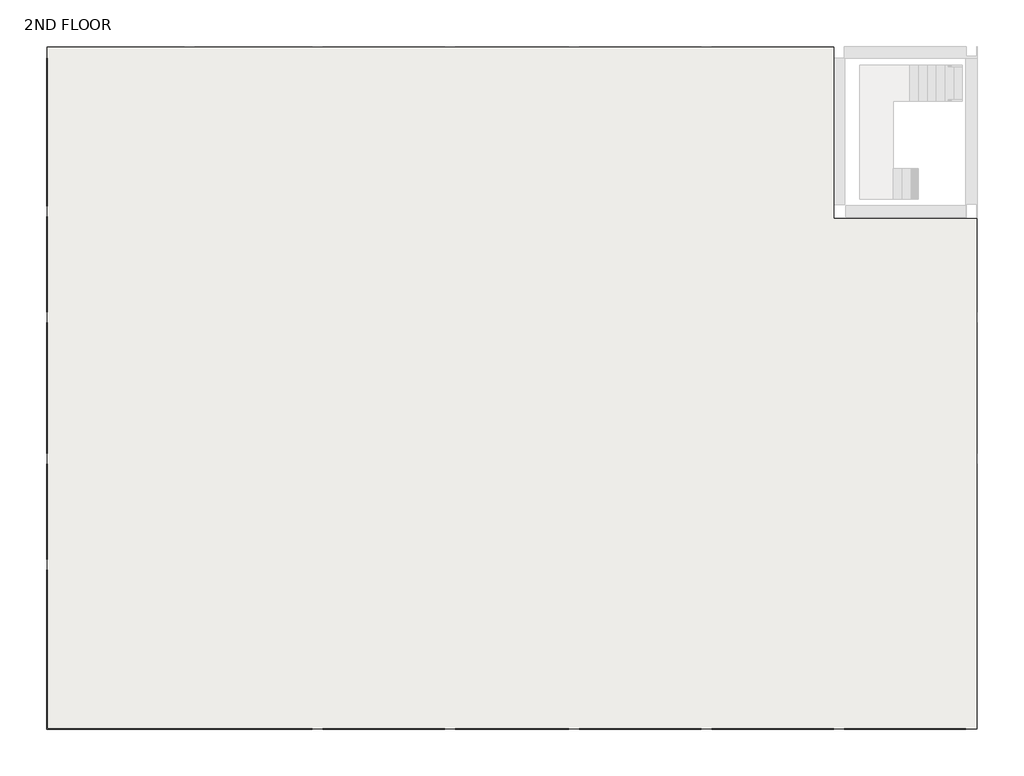
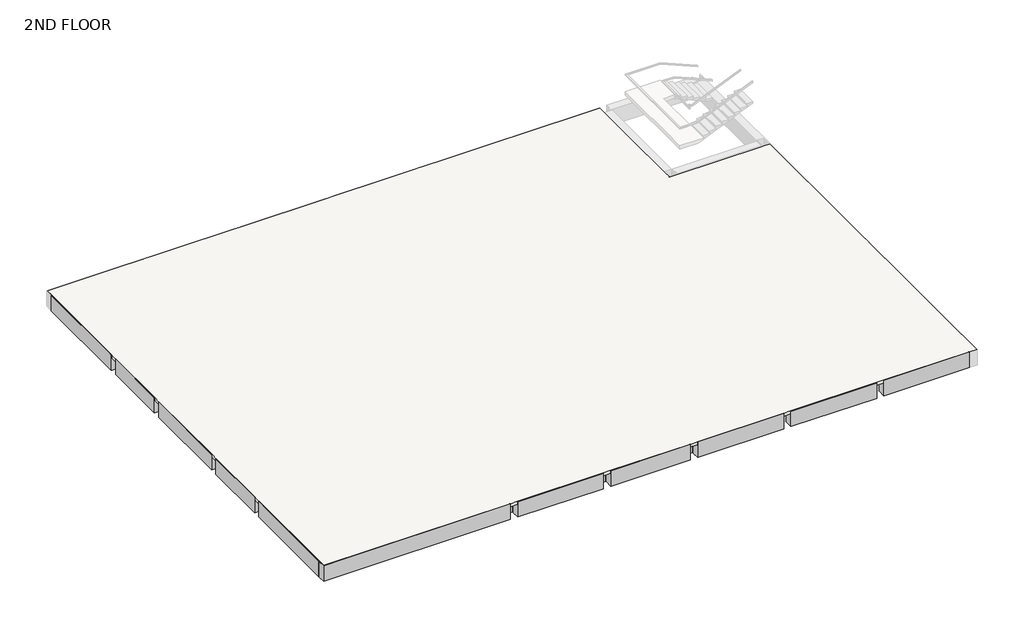
# One storey, part 1 of 2: 9 beams, 1 slab.
"""IFC4 building model written with IfcOpenShell, lengths in millimetres."""

from ifc_helpers import new_model, si_unit, frame, origin, place, context, project, spatial, polyline, outline, extrude, faceted_brep, element, save

model = new_model("IFC4")

# Units and contexts
model_context = context("Model", 3, world=origin())
ifc_project = project(units=[si_unit("LENGTHUNIT", "METRE", prefix="MILLI")], contexts=[model_context])

# Site, building, storey
site = spatial("IfcSite", under=ifc_project)
building = spatial("IfcBuilding", under=site)
storey = spatial("IfcBuildingStorey", under=building, Name="2ND FLOOR", Elevation=7620.0)

# Beams
placement = place(None, origin())
element("IfcBeam", 1, ObjectType="M_Concrete-Rectangular Beam : 400 x 800mm", at=placement, inside=storey, context=model_context, shape_type="Brep", body=[
    faceted_brep([(-25701.5491019, -6047.8309165, 7620.0), (-25701.5491019, -6447.8309165, 7620.0), (-16535.3491019, -6447.8309165, 7620.0), (-16535.3491019, -6425.6309165, 7620.0), (-25679.3491019, -6425.6309165, 7620.0), (-25679.3491019, -6047.8309165, 7620.0), (-25701.5491019, -6047.8309165, 6820.0), (-25679.3491019, -6047.8309165, 7467.6), (-25301.5491019, -6047.8309165, 7467.6), (-20977.1491019, -6047.8309165, 7467.6), (-20577.1491019, -6047.8309165, 7467.6), (-16557.5491019, -6047.8309165, 7467.6), (-16535.3491019, -6047.8309165, 7467.6), (-16535.3491019, -6047.8309165, 6820.0), (-16557.5491019, -6047.8309165, 6820.0), (-20577.1491019, -6047.8309165, 6820.0), (-20977.1491019, -6047.8309165, 6820.0), (-25301.5491019, -6047.8309165, 6820.0), (-25701.5491019, -6447.8309165, 6820.0), (-16535.3491019, -6447.8309165, 6820.0), (-25323.7491019, -6425.6309165, 6820.0), (-25323.7491019, -6070.0309165, 6820.0), (-25679.3491019, -6070.0309165, 6820.0), (-25679.3491019, -6425.6309165, 6820.0), (-20599.3491019, -6425.6309165, 6820.0), (-20599.3491019, -6070.0309165, 6820.0), (-20954.9491019, -6070.0309165, 6820.0), (-20954.9491019, -6425.6309165, 6820.0), (-25323.7491019, -6425.6309165, 7467.6), (-25323.7491019, -6070.0309165, 7467.6), (-16535.3491019, -6425.6309165, 7467.6), (-20599.3491019, -6425.6309165, 7467.6), (-20954.9491019, -6425.6309165, 7467.6), (-25679.3491019, -6425.6309165, 7467.6), (-25679.3491019, -6070.0309165, 7467.6), (-20599.3491019, -6070.0309165, 7467.6), (-20954.9491019, -6070.0309165, 7467.6)], [[[0, 1, 2, 3, 4, 5]], [[6, 0, 5, 7, 8, 9, 10, 11, 12, 13, 14, 15, 16, 17]], [[18, 6, 17, 16, 15, 14, 13, 19], [20, 21, 22, 23], [24, 25, 26, 27]], [[1, 18, 19, 2]], [[1, 0, 6, 18]], [[21, 20, 28, 29]], [[30, 31, 24, 27, 32, 28, 20, 23, 33, 4, 3]], [[4, 33, 23, 22, 34, 7, 5]], [[22, 21, 29, 34]], [[25, 24, 31, 35]], [[27, 26, 36, 32]], [[26, 25, 35, 36]], [[19, 13, 12, 30, 3, 2]], [[28, 32, 36, 35, 31, 30, 12, 11, 10, 9, 8, 7, 34, 29]]]),
    faceted_brep([(5997.6508981, -6447.8309165, 6820.0), (5997.6508981, -6047.8309165, 6820.0), (5997.6508981, -6047.8309165, 7467.6), (5997.6508981, -6425.6309165, 7467.6), (5997.6508981, -6425.6309165, 7620.0), (5997.6508981, -6447.8309165, 7620.0), (1803.4508981, -6047.8309165, 6820.0), (1803.4508981, -6447.8309165, 6820.0), (1803.4508981, -6447.8309165, 7620.0), (1803.4508981, -6425.6309165, 7620.0), (1803.4508981, -6425.6309165, 7467.6), (1803.4508981, -6047.8309165, 7467.6), (1825.6508981, -6047.8309165, 6820.0), (1825.6508981, -6047.8309165, 7467.6)], [[[0, 1, 2, 3, 4, 5]], [[6, 7, 8, 9, 10, 11]], [[8, 5, 4, 9]], [[1, 12, 6, 11, 13, 2]], [[1, 0, 7, 6, 12]], [[0, 5, 8, 7]], [[10, 3, 2, 13, 11]], [[3, 10, 9, 4]]]),
    faceted_brep([(-16179.7491019, -6047.8309165, 6820.0), (-16179.7491019, -6447.8309165, 6820.0), (-16179.7491019, -6447.8309165, 7620.0), (-16179.7491019, -6425.6309165, 7620.0), (-16179.7491019, -6425.6309165, 7467.6), (-16179.7491019, -6047.8309165, 7467.6), (-11963.3491019, -6447.8309165, 7620.0), (-11963.3491019, -6425.6309165, 7620.0), (-11963.3491019, -6047.8309165, 6820.0), (-11985.5491019, -6047.8309165, 6820.0), (-16157.5491019, -6047.8309165, 6820.0), (-16157.5491019, -6047.8309165, 7467.6), (-11985.5491019, -6047.8309165, 7467.6), (-11963.3491019, -6047.8309165, 7467.6), (-11963.3491019, -6447.8309165, 6820.0), (-11963.3491019, -6425.6309165, 7467.6)], [[[0, 1, 2, 3, 4, 5]], [[2, 6, 7, 3]], [[8, 9, 10, 0, 5, 11, 12, 13]], [[1, 0, 10, 9, 8, 14]], [[2, 1, 14, 6]], [[14, 8, 13, 15, 7, 6]], [[15, 4, 3, 7]], [[4, 15, 13, 12, 11, 5]]]),
    faceted_brep([(-11607.7491019, -6047.8309165, 6820.0), (-11607.7491019, -6447.8309165, 6820.0), (-11607.7491019, -6447.8309165, 7620.0), (-11607.7491019, -6425.6309165, 7620.0), (-11607.7491019, -6425.6309165, 7467.6), (-11607.7491019, -6047.8309165, 7467.6), (-7696.1491019, -6447.8309165, 7620.0), (-7696.1491019, -6425.6309165, 7620.0), (-7696.1491019, -6047.8309165, 6820.0), (-7718.3491019, -6047.8309165, 6820.0), (-11585.5491019, -6047.8309165, 6820.0), (-11585.5491019, -6047.8309165, 7467.6), (-7718.3491019, -6047.8309165, 7467.6), (-7696.1491019, -6047.8309165, 7467.6), (-7696.1491019, -6447.8309165, 6820.0), (-7696.1491019, -6425.6309165, 7467.6)], [[[0, 1, 2, 3, 4, 5]], [[2, 6, 7, 3]], [[8, 9, 10, 0, 5, 11, 12, 13]], [[1, 0, 10, 9, 8, 14]], [[2, 1, 14, 6]], [[14, 8, 13, 15, 7, 6]], [[15, 4, 3, 7]], [[4, 15, 13, 12, 11, 5]]]),
    faceted_brep([(-7340.5491019, -6047.8309165, 6820.0), (-7340.5491019, -6447.8309165, 6820.0), (-7340.5491019, -6447.8309165, 7620.0), (-7340.5491019, -6425.6309165, 7620.0), (-7340.5491019, -6425.6309165, 7467.6), (-7340.5491019, -6047.8309165, 7467.6), (-3124.1491019, -6447.8309165, 7620.0), (-3124.1491019, -6425.6309165, 7620.0), (-3124.1491019, -6047.8309165, 6820.0), (-3146.3491019, -6047.8309165, 6820.0), (-7318.3491019, -6047.8309165, 6820.0), (-7318.3491019, -6047.8309165, 7467.6), (-3146.3491019, -6047.8309165, 7467.6), (-3124.1491019, -6047.8309165, 7467.6), (-3124.1491019, -6447.8309165, 6820.0), (-3124.1491019, -6425.6309165, 7467.6)], [[[0, 1, 2, 3, 4, 5]], [[2, 6, 7, 3]], [[8, 9, 10, 0, 5, 11, 12, 13]], [[1, 0, 10, 9, 8, 14]], [[2, 1, 14, 6]], [[14, 8, 13, 15, 7, 6]], [[15, 4, 3, 7]], [[4, 15, 13, 12, 11, 5]]]),
    faceted_brep([(-2768.5491019, -6047.8309165, 6820.0), (-2768.5491019, -6447.8309165, 6820.0), (-2768.5491019, -6447.8309165, 7620.0), (-2768.5491019, -6425.6309165, 7620.0), (-2768.5491019, -6425.6309165, 7467.6), (-2768.5491019, -6047.8309165, 7467.6), (1447.8508981, -6447.8309165, 7620.0), (1447.8508981, -6425.6309165, 7620.0), (1447.8508981, -6047.8309165, 6820.0), (1425.6508981, -6047.8309165, 6820.0), (-2746.3491019, -6047.8309165, 6820.0), (-2746.3491019, -6047.8309165, 7467.6), (1425.6508981, -6047.8309165, 7467.6), (1447.8508981, -6047.8309165, 7467.6), (1447.8508981, -6447.8309165, 6820.0), (1447.8508981, -6425.6309165, 7467.6)], [[[0, 1, 2, 3, 4, 5]], [[2, 6, 7, 3]], [[8, 9, 10, 0, 5, 11, 12, 13]], [[1, 0, 10, 9, 8, 14]], [[2, 1, 14, 6]], [[14, 8, 13, 15, 7, 6]], [[15, 4, 3, 7]], [[4, 15, 13, 12, 11, 5]]]),
])
element("IfcBeam", 2, ObjectType="M_Concrete-Rectangular Beam : 400 x 800mm", at=placement, inside=storey, context=model_context, shape_type="Brep", body=[
    faceted_brep([(-25701.5491019, -939.2309165, 7620.0), (-25701.5491019, -6047.8309165, 7620.0), (-25679.3491019, -6047.8309165, 7620.0), (-25679.3491019, -939.2309165, 7620.0), (-25301.5491019, -6047.8309165, 6820.0), (-25301.5491019, -961.4309165, 6820.0), (-25301.5491019, -939.2309165, 6820.0), (-25301.5491019, -939.2309165, 7467.6), (-25301.5491019, -961.4309165, 7467.6), (-25301.5491019, -6047.8309165, 7467.6), (-25701.5491019, -6047.8309165, 6820.0), (-25701.5491019, -939.2309165, 6820.0), (-25679.3491019, -6047.8309165, 7467.6), (-25679.3491019, -939.2309165, 7467.6)], [[[0, 1, 2, 3]], [[4, 5, 6, 7, 8, 9]], [[4, 10, 11, 6, 5]], [[10, 1, 0, 11]], [[10, 4, 9, 12, 2, 1]], [[6, 11, 0, 3, 13, 7]], [[12, 13, 3, 2]], [[13, 12, 9, 8, 7]]]),
    faceted_brep([(-25301.5491019, 16716.9690835, 6820.0), (-25701.5491019, 16716.9690835, 6820.0), (-25701.5491019, 16716.9690835, 7620.0), (-25679.3491019, 16716.9690835, 7620.0), (-25679.3491019, 16716.9690835, 7467.6), (-25301.5491019, 16716.9690835, 7467.6), (-25701.5491019, 11608.3690835, 7620.0), (-25679.3491019, 11608.3690835, 7620.0), (-25301.5491019, 11608.3690835, 6820.0), (-25301.5491019, 11630.5690835, 6820.0), (-25301.5491019, 11630.5690835, 7467.6), (-25301.5491019, 11608.3690835, 7467.6), (-25701.5491019, 11608.3690835, 6820.0), (-25679.3491019, 11608.3690835, 7467.6)], [[[0, 1, 2, 3, 4, 5]], [[2, 6, 7, 3]], [[8, 9, 0, 5, 10, 11]], [[1, 0, 9, 8, 12]], [[2, 1, 12, 6]], [[12, 8, 11, 13, 7, 6]], [[4, 13, 11, 10, 5]], [[13, 4, 3, 7]]]),
    faceted_brep([(-25701.5491019, 7950.7690835, 6820.0), (-25301.5491019, 7950.7690835, 6820.0), (-25301.5491019, 7950.7690835, 7467.6), (-25679.3491019, 7950.7690835, 7467.6), (-25679.3491019, 7950.7690835, 7620.0), (-25701.5491019, 7950.7690835, 7620.0), (-25301.5491019, 11252.7690835, 6820.0), (-25701.5491019, 11252.7690835, 6820.0), (-25701.5491019, 11252.7690835, 7620.0), (-25679.3491019, 11252.7690835, 7620.0), (-25679.3491019, 11252.7690835, 7467.6), (-25301.5491019, 11252.7690835, 7467.6), (-25301.5491019, 7972.9690835, 7467.6), (-25301.5491019, 11230.5690835, 7467.6), (-25301.5491019, 7972.9690835, 6820.0), (-25301.5491019, 11230.5690835, 6820.0)], [[[0, 1, 2, 3, 4, 5]], [[6, 7, 8, 9, 10, 11]], [[10, 3, 2, 12, 13, 11]], [[3, 10, 9, 4]], [[8, 5, 4, 9]], [[1, 14, 15, 6, 11, 13, 12, 2]], [[1, 0, 7, 6, 15, 14]], [[0, 5, 8, 7]]]),
    faceted_brep([(-25301.5491019, 7595.1690835, 6820.0), (-25701.5491019, 7595.1690835, 6820.0), (-25701.5491019, 7595.1690835, 7620.0), (-25679.3491019, 7595.1690835, 7620.0), (-25679.3491019, 7595.1690835, 7467.6), (-25301.5491019, 7595.1690835, 7467.6), (-25701.5491019, 3073.9690835, 6820.0), (-25301.5491019, 3073.9690835, 6820.0), (-25301.5491019, 3073.9690835, 7467.6), (-25679.3491019, 3073.9690835, 7467.6), (-25679.3491019, 3073.9690835, 7620.0), (-25701.5491019, 3073.9690835, 7620.0), (-25301.5491019, 3096.1690835, 7467.6), (-25301.5491019, 7572.9690835, 7467.6), (-25301.5491019, 3096.1690835, 6820.0), (-25301.5491019, 7572.9690835, 6820.0)], [[[0, 1, 2, 3, 4, 5]], [[6, 7, 8, 9, 10, 11]], [[4, 9, 8, 12, 13, 5]], [[9, 4, 3, 10]], [[2, 11, 10, 3]], [[7, 14, 15, 0, 5, 13, 12, 8]], [[1, 0, 15, 14, 7, 6]], [[2, 1, 6, 11]]]),
    faceted_brep([(-25301.5491019, 2718.3690835, 6820.0), (-25701.5491019, 2718.3690835, 6820.0), (-25701.5491019, 2718.3690835, 7620.0), (-25679.3491019, 2718.3690835, 7620.0), (-25679.3491019, 2718.3690835, 7467.6), (-25301.5491019, 2718.3690835, 7467.6), (-25701.5491019, -583.6309165, 6820.0), (-25301.5491019, -583.6309165, 6820.0), (-25301.5491019, -583.6309165, 7467.6), (-25679.3491019, -583.6309165, 7467.6), (-25679.3491019, -583.6309165, 7620.0), (-25701.5491019, -583.6309165, 7620.0), (-25301.5491019, -561.4309165, 7467.6), (-25301.5491019, 2696.1690835, 7467.6), (-25301.5491019, -561.4309165, 6820.0), (-25301.5491019, 2696.1690835, 6820.0)], [[[0, 1, 2, 3, 4, 5]], [[6, 7, 8, 9, 10, 11]], [[4, 9, 8, 12, 13, 5]], [[9, 4, 3, 10]], [[2, 11, 10, 3]], [[7, 14, 15, 0, 5, 13, 12, 8]], [[0, 15, 14, 7, 6, 1]], [[11, 2, 1, 6]]]),
])
element("IfcBeam", 3, ObjectType="M_Concrete-Rectangular Beam : 400 x 800mm", at=placement, inside=storey, context=model_context, shape_type="SweptSolid", body=[
    extrude(outline(polyline([(-20577.1491019, -6047.8309165), (-20977.1491019, -6047.8309165), (-20977.1491019, -990.0309165), (-20577.1491019, -990.0309165), (-20577.1491019, -6047.8309165)])), frame((0.0, 0.0, 6820.0), z_axis=(0.0, 0.0, 1.0), x_axis=(1.0, 0.0, 0.0)), (0.0, 0.0, 1.0), 647.6),
    extrude(outline(polyline([(-20599.3491019, 16716.9690835), (-20577.1491019, 16716.9690835), (-20577.1491019, 11659.1690835), (-20977.1491019, 11659.1690835), (-20977.1491019, 16716.9690835), (-20954.9491019, 16716.9690835), (-20954.9491019, 16662.9690835), (-20599.3491019, 16662.9690835), (-20599.3491019, 16716.9690835)])), frame((0.0, 0.0, 6820.0), z_axis=(0.0, 0.0, 1.0), x_axis=(1.0, 0.0, 0.0)), (0.0, 0.0, 1.0), 647.6),
    extrude(outline(polyline([(-20977.1491019, 11201.9690835), (-20577.1491019, 11201.9690835), (-20577.1491019, 8001.5690835), (-20977.1491019, 8001.5690835), (-20977.1491019, 11201.9690835)])), frame((0.0, 0.0, 6820.0), z_axis=(0.0, 0.0, 1.0), x_axis=(1.0, 0.0, 0.0)), (0.0, 0.0, 1.0), 647.6),
    extrude(outline(polyline([(-20977.1491019, 7544.3690835), (-20577.1491019, 7544.3690835), (-20577.1491019, 3124.7690835), (-20977.1491019, 3124.7690835), (-20977.1491019, 7544.3690835)])), frame((0.0, 0.0, 6820.0), z_axis=(0.0, 0.0, 1.0), x_axis=(1.0, 0.0, 0.0)), (0.0, 0.0, 1.0), 647.6),
    extrude(outline(polyline([(-20977.1491019, 2667.5690835), (-20577.1491019, 2667.5690835), (-20577.1491019, -532.8309165), (-20977.1491019, -532.8309165), (-20977.1491019, 2667.5690835)])), frame((0.0, 0.0, 6820.0), z_axis=(0.0, 0.0, 1.0), x_axis=(1.0, 0.0, 0.0)), (0.0, 0.0, 1.0), 647.6),
])
element("IfcBeam", 4, ObjectType="M_Concrete-Rectangular Beam : 400 x 800mm", at=placement, inside=storey, context=model_context, shape_type="SweptSolid", body=[
    extrude(outline(polyline([(-16157.5491019, -6047.8309165), (-16179.7491019, -6047.8309165), (-16179.7491019, -6019.2309165), (-16535.3491019, -6019.2309165), (-16535.3491019, -6047.8309165), (-16557.5491019, -6047.8309165), (-16557.5491019, -990.0309165), (-16157.5491019, -990.0309165), (-16157.5491019, -6047.8309165)])), frame((0.0, 0.0, 6820.0), z_axis=(0.0, 0.0, 1.0), x_axis=(1.0, 0.0, 0.0)), (0.0, 0.0, 1.0), 647.6),
    extrude(outline(polyline([(-16179.7491019, 16716.9690835), (-16157.5491019, 16716.9690835), (-16157.5491019, 11659.1690835), (-16557.5491019, 11659.1690835), (-16557.5491019, 16716.9690835), (-16535.3491019, 16716.9690835), (-16535.3491019, 16688.3690835), (-16179.7491019, 16688.3690835), (-16179.7491019, 16716.9690835)])), frame((0.0, 0.0, 6820.0), z_axis=(0.0, 0.0, 1.0), x_axis=(1.0, 0.0, 0.0)), (0.0, 0.0, 1.0), 647.6),
    extrude(outline(polyline([(-16557.5491019, 11201.9690835), (-16157.5491019, 11201.9690835), (-16157.5491019, 8001.5690835), (-16557.5491019, 8001.5690835), (-16557.5491019, 11201.9690835)])), frame((0.0, 0.0, 6820.0), z_axis=(0.0, 0.0, 1.0), x_axis=(1.0, 0.0, 0.0)), (0.0, 0.0, 1.0), 647.6),
    extrude(outline(polyline([(-16557.5491019, 7544.3690835), (-16157.5491019, 7544.3690835), (-16157.5491019, 3124.7690835), (-16557.5491019, 3124.7690835), (-16557.5491019, 7544.3690835)])), frame((0.0, 0.0, 6820.0), z_axis=(0.0, 0.0, 1.0), x_axis=(1.0, 0.0, 0.0)), (0.0, 0.0, 1.0), 647.6),
    extrude(outline(polyline([(-16557.5491019, 2667.5690835), (-16157.5491019, 2667.5690835), (-16157.5491019, -532.8309165), (-16557.5491019, -532.8309165), (-16557.5491019, 2667.5690835)])), frame((0.0, 0.0, 6820.0), z_axis=(0.0, 0.0, 1.0), x_axis=(1.0, 0.0, 0.0)), (0.0, 0.0, 1.0), 647.6),
])
element("IfcBeam", 5, ObjectType="M_Concrete-Rectangular Beam : 400 x 800mm", at=placement, inside=storey, context=model_context, shape_type="SweptSolid", body=[
    extrude(outline(polyline([(-11585.5491019, -6047.8309165), (-11607.7491019, -6047.8309165), (-11607.7491019, -6019.2309165), (-11963.3491019, -6019.2309165), (-11963.3491019, -6047.8309165), (-11985.5491019, -6047.8309165), (-11985.5491019, -990.0309165), (-11585.5491019, -990.0309165), (-11585.5491019, -6047.8309165)])), frame((0.0, 0.0, 6820.0), z_axis=(0.0, 0.0, 1.0), x_axis=(1.0, 0.0, 0.0)), (0.0, 0.0, 1.0), 647.6),
    extrude(outline(polyline([(-11607.7491019, 16716.9690835), (-11585.5491019, 16716.9690835), (-11585.5491019, 11659.1690835), (-11985.5491019, 11659.1690835), (-11985.5491019, 16716.9690835), (-11963.3491019, 16716.9690835), (-11963.3491019, 16688.3690835), (-11607.7491019, 16688.3690835), (-11607.7491019, 16716.9690835)])), frame((0.0, 0.0, 6820.0), z_axis=(0.0, 0.0, 1.0), x_axis=(1.0, 0.0, 0.0)), (0.0, 0.0, 1.0), 647.6),
    extrude(outline(polyline([(-11985.5491019, 11201.9690835), (-11585.5491019, 11201.9690835), (-11585.5491019, 8001.5690835), (-11985.5491019, 8001.5690835), (-11985.5491019, 11201.9690835)])), frame((0.0, 0.0, 6820.0), z_axis=(0.0, 0.0, 1.0), x_axis=(1.0, 0.0, 0.0)), (0.0, 0.0, 1.0), 647.6),
    extrude(outline(polyline([(-11985.5491019, 7544.3690835), (-11585.5491019, 7544.3690835), (-11585.5491019, 3124.7690835), (-11985.5491019, 3124.7690835), (-11985.5491019, 7544.3690835)])), frame((0.0, 0.0, 6820.0), z_axis=(0.0, 0.0, 1.0), x_axis=(1.0, 0.0, 0.0)), (0.0, 0.0, 1.0), 647.6),
    extrude(outline(polyline([(-11585.5491019, -532.8309165), (-11985.5491019, -532.8309165), (-11985.5491019, 2667.5690835), (-11585.5491019, 2667.5690835), (-11585.5491019, -532.8309165)])), frame((0.0, 0.0, 6820.0), z_axis=(0.0, 0.0, 1.0), x_axis=(1.0, 0.0, 0.0)), (0.0, 0.0, 1.0), 647.6),
])
element("IfcBeam", 6, ObjectType="M_Concrete-Rectangular Beam : 400 x 800mm", at=placement, inside=storey, context=model_context, shape_type="SweptSolid", body=[
    extrude(outline(polyline([(-7318.3491019, -6047.8309165), (-7340.5491019, -6047.8309165), (-7340.5491019, -6019.2309165), (-7696.1491019, -6019.2309165), (-7696.1491019, -6047.8309165), (-7718.3491019, -6047.8309165), (-7718.3491019, -990.0309165), (-7318.3491019, -990.0309165), (-7318.3491019, -6047.8309165)])), frame((0.0, 0.0, 6820.0), z_axis=(0.0, 0.0, 1.0), x_axis=(1.0, 0.0, 0.0)), (0.0, 0.0, 1.0), 647.6),
    extrude(outline(polyline([(-7340.5491019, 16716.9690835), (-7318.3491019, 16716.9690835), (-7318.3491019, 11659.1690835), (-7718.3491019, 11659.1690835), (-7718.3491019, 16716.9690835), (-7696.1491019, 16716.9690835), (-7696.1491019, 16688.3690835), (-7340.5491019, 16688.3690835), (-7340.5491019, 16716.9690835)])), frame((0.0, 0.0, 6820.0), z_axis=(0.0, 0.0, 1.0), x_axis=(1.0, 0.0, 0.0)), (0.0, 0.0, 1.0), 647.6),
    extrude(outline(polyline([(-7718.3491019, 7544.3690835), (-7318.3491019, 7544.3690835), (-7318.3491019, 3124.7690835), (-7718.3491019, 3124.7690835), (-7718.3491019, 7544.3690835)])), frame((0.0, 0.0, 6820.0), z_axis=(0.0, 0.0, 1.0), x_axis=(1.0, 0.0, 0.0)), (0.0, 0.0, 1.0), 647.6),
    extrude(outline(polyline([(-7318.3491019, 8001.5690835), (-7718.3491019, 8001.5690835), (-7718.3491019, 11201.9690835), (-7318.3491019, 11201.9690835), (-7318.3491019, 8001.5690835)])), frame((0.0, 0.0, 6820.0), z_axis=(0.0, 0.0, 1.0), x_axis=(1.0, 0.0, 0.0)), (0.0, 0.0, 1.0), 647.6),
    extrude(outline(polyline([(-7318.3491019, -532.8309165), (-7718.3491019, -532.8309165), (-7718.3491019, 2667.5690835), (-7318.3491019, 2667.5690835), (-7318.3491019, -532.8309165)])), frame((0.0, 0.0, 6820.0), z_axis=(0.0, 0.0, 1.0), x_axis=(1.0, 0.0, 0.0)), (0.0, 0.0, 1.0), 647.6),
])
element("IfcBeam", 7, ObjectType="M_Concrete-Rectangular Beam : 400 x 800mm", at=placement, inside=storey, context=model_context, shape_type="SweptSolid", body=[
    extrude(outline(polyline([(-25301.5491019, 3073.9690835), (-25301.5491019, 3096.1690835), (-21005.7491019, 3096.1690835), (-21005.7491019, 2696.1690835), (-25301.5491019, 2696.1690835), (-25301.5491019, 2718.3690835), (-25272.9491019, 2718.3690835), (-25272.9491019, 3073.9690835), (-25301.5491019, 3073.9690835)])), frame((0.0, 0.0, 6820.0), z_axis=(0.0, 0.0, 1.0), x_axis=(1.0, 0.0, 0.0)), (0.0, 0.0, 1.0), 647.6),
    extrude(outline(polyline([(5997.6508981, 3096.1690835), (5997.6508981, 3073.9690835), (5969.0508981, 3073.9690835), (5969.0508981, 2718.3690835), (5997.6508981, 2718.3690835), (5997.6508981, 2696.1690835), (1854.2508981, 2696.1690835), (1854.2508981, 3096.1690835), (5997.6508981, 3096.1690835)])), frame((0.0, 0.0, 6820.0), z_axis=(0.0, 0.0, 1.0), x_axis=(1.0, 0.0, 0.0)), (0.0, 0.0, 1.0), 647.6),
    extrude(outline(polyline([(-20548.5491019, 2696.1690835), (-20548.5491019, 3096.1690835), (-16586.1491019, 3096.1690835), (-16586.1491019, 2696.1690835), (-20548.5491019, 2696.1690835)])), frame((0.0, 0.0, 6820.0), z_axis=(0.0, 0.0, 1.0), x_axis=(1.0, 0.0, 0.0)), (0.0, 0.0, 1.0), 647.6),
    extrude(outline(polyline([(-16128.9491019, 2696.1690835), (-16128.9491019, 3096.1690835), (-12014.1491019, 3096.1690835), (-12014.1491019, 2696.1690835), (-16128.9491019, 2696.1690835)])), frame((0.0, 0.0, 6820.0), z_axis=(0.0, 0.0, 1.0), x_axis=(1.0, 0.0, 0.0)), (0.0, 0.0, 1.0), 647.6),
    extrude(outline(polyline([(1397.0508981, 3096.1690835), (1397.0508981, 2696.1690835), (-2717.7491019, 2696.1690835), (-2717.7491019, 3096.1690835), (1397.0508981, 3096.1690835)])), frame((0.0, 0.0, 6820.0), z_axis=(0.0, 0.0, 1.0), x_axis=(1.0, 0.0, 0.0)), (0.0, 0.0, 1.0), 647.6),
    extrude(outline(polyline([(-3174.9491019, 3096.1690835), (-3174.9491019, 2696.1690835), (-7289.7491019, 2696.1690835), (-7289.7491019, 3096.1690835), (-3174.9491019, 3096.1690835)])), frame((0.0, 0.0, 6820.0), z_axis=(0.0, 0.0, 1.0), x_axis=(1.0, 0.0, 0.0)), (0.0, 0.0, 1.0), 647.6),
    extrude(outline(polyline([(-7746.9491019, 3096.1690835), (-7746.9491019, 2696.1690835), (-11556.9491019, 2696.1690835), (-11556.9491019, 3096.1690835), (-7746.9491019, 3096.1690835)])), frame((0.0, 0.0, 6820.0), z_axis=(0.0, 0.0, 1.0), x_axis=(1.0, 0.0, 0.0)), (0.0, 0.0, 1.0), 647.6),
])
element("IfcBeam", 8, ObjectType="M_Concrete-Rectangular Beam : 400 x 800mm", at=placement, inside=storey, context=model_context, shape_type="SweptSolid", body=[
    extrude(outline(polyline([(-25301.5491019, -583.6309165), (-25301.5491019, -561.4309165), (-21005.7491019, -561.4309165), (-21005.7491019, -961.4309165), (-25301.5491019, -961.4309165), (-25301.5491019, -939.2309165), (-25247.5491019, -939.2309165), (-25247.5491019, -583.6309165), (-25301.5491019, -583.6309165)])), frame((0.0, 0.0, 6820.0), z_axis=(0.0, 0.0, 1.0), x_axis=(1.0, 0.0, 0.0)), (0.0, 0.0, 1.0), 647.6),
    extrude(outline(polyline([(5997.6508981, -561.4309165), (5997.6508981, -961.4309165), (1854.2508981, -961.4309165), (1854.2508981, -561.4309165), (5997.6508981, -561.4309165)])), frame((0.0, 0.0, 6820.0), z_axis=(0.0, 0.0, 1.0), x_axis=(1.0, 0.0, 0.0)), (0.0, 0.0, 1.0), 647.6),
    extrude(outline(polyline([(-20548.5491019, -961.4309165), (-20548.5491019, -561.4309165), (-16586.1491019, -561.4309165), (-16586.1491019, -961.4309165), (-20548.5491019, -961.4309165)])), frame((0.0, 0.0, 6820.0), z_axis=(0.0, 0.0, 1.0), x_axis=(1.0, 0.0, 0.0)), (0.0, 0.0, 1.0), 647.6),
    extrude(outline(polyline([(-16128.9491019, -961.4309165), (-16128.9491019, -561.4309165), (-12014.1491019, -561.4309165), (-12014.1491019, -961.4309165), (-16128.9491019, -961.4309165)])), frame((0.0, 0.0, 6820.0), z_axis=(0.0, 0.0, 1.0), x_axis=(1.0, 0.0, 0.0)), (0.0, 0.0, 1.0), 647.6),
    extrude(outline(polyline([(-11556.9491019, -961.4309165), (-11556.9491019, -561.4309165), (-7746.9491019, -561.4309165), (-7746.9491019, -961.4309165), (-11556.9491019, -961.4309165)])), frame((0.0, 0.0, 6820.0), z_axis=(0.0, 0.0, 1.0), x_axis=(1.0, 0.0, 0.0)), (0.0, 0.0, 1.0), 647.6),
    extrude(outline(polyline([(-7289.7491019, -961.4309165), (-7289.7491019, -561.4309165), (-3174.9491019, -561.4309165), (-3174.9491019, -961.4309165), (-7289.7491019, -961.4309165)])), frame((0.0, 0.0, 6820.0), z_axis=(0.0, 0.0, 1.0), x_axis=(1.0, 0.0, 0.0)), (0.0, 0.0, 1.0), 647.6),
    extrude(outline(polyline([(-2717.7491019, -961.4309165), (-2717.7491019, -561.4309165), (1397.0508981, -561.4309165), (1397.0508981, -961.4309165), (-2717.7491019, -961.4309165)])), frame((0.0, 0.0, 6820.0), z_axis=(0.0, 0.0, 1.0), x_axis=(1.0, 0.0, 0.0)), (0.0, 0.0, 1.0), 647.6),
])
element("IfcBeam", 9, ObjectType="M_Concrete-Rectangular Beam : 400 x 800mm", at=placement, inside=storey, context=model_context, shape_type="SweptSolid", body=[
    extrude(outline(polyline([(-25301.5491019, 7950.7690835), (-25301.5491019, 7972.9690835), (-21005.7491019, 7972.9690835), (-21005.7491019, 7572.9690835), (-25301.5491019, 7572.9690835), (-25301.5491019, 7595.1690835), (-25272.9491019, 7595.1690835), (-25272.9491019, 7950.7690835), (-25301.5491019, 7950.7690835)])), frame((0.0, 0.0, 6820.0), z_axis=(0.0, 0.0, 1.0), x_axis=(1.0, 0.0, 0.0)), (0.0, 0.0, 1.0), 647.6),
    extrude(outline(polyline([(5997.6508981, 7972.9690835), (5997.6508981, 7950.7690835), (5969.0508981, 7950.7690835), (5969.0508981, 7595.1690835), (5997.6508981, 7595.1690835), (5997.6508981, 7572.9690835), (1854.2508981, 7572.9690835), (1854.2508981, 7972.9690835), (5997.6508981, 7972.9690835)])), frame((0.0, 0.0, 6820.0), z_axis=(0.0, 0.0, 1.0), x_axis=(1.0, 0.0, 0.0)), (0.0, 0.0, 1.0), 647.6),
    extrude(outline(polyline([(-7289.7491019, 7572.9690835), (-7289.7491019, 7972.9690835), (-3174.9491019, 7972.9690835), (-3174.9491019, 7572.9690835), (-7289.7491019, 7572.9690835)])), frame((0.0, 0.0, 6820.0), z_axis=(0.0, 0.0, 1.0), x_axis=(1.0, 0.0, 0.0)), (0.0, 0.0, 1.0), 647.6),
    extrude(outline(polyline([(-7746.9491019, 7972.9690835), (-7746.9491019, 7572.9690835), (-11556.9491019, 7572.9690835), (-11556.9491019, 7972.9690835), (-7746.9491019, 7972.9690835)])), frame((0.0, 0.0, 6820.0), z_axis=(0.0, 0.0, 1.0), x_axis=(1.0, 0.0, 0.0)), (0.0, 0.0, 1.0), 647.6),
    extrude(outline(polyline([(1397.0508981, 7972.9690835), (1397.0508981, 7572.9690835), (-2717.7491019, 7572.9690835), (-2717.7491019, 7972.9690835), (1397.0508981, 7972.9690835)])), frame((0.0, 0.0, 6820.0), z_axis=(0.0, 0.0, 1.0), x_axis=(1.0, 0.0, 0.0)), (0.0, 0.0, 1.0), 647.6),
    extrude(outline(polyline([(-12014.1491019, 7972.9690835), (-12014.1491019, 7572.9690835), (-16128.9491019, 7572.9690835), (-16128.9491019, 7972.9690835), (-12014.1491019, 7972.9690835)])), frame((0.0, 0.0, 6820.0), z_axis=(0.0, 0.0, 1.0), x_axis=(1.0, 0.0, 0.0)), (0.0, 0.0, 1.0), 647.6),
    extrude(outline(polyline([(-16586.1491019, 7972.9690835), (-16586.1491019, 7572.9690835), (-20548.5491019, 7572.9690835), (-20548.5491019, 7972.9690835), (-16586.1491019, 7972.9690835)])), frame((0.0, 0.0, 6820.0), z_axis=(0.0, 0.0, 1.0), x_axis=(1.0, 0.0, 0.0)), (0.0, 0.0, 1.0), 647.6),
])

# Slab
element("IfcSlab", 10, ObjectType="6\" Foundation Slab", at=placement, inside=storey, context=model_context, shape_type="Brep", body=[
    faceted_brep([(6375.4508981, -6425.6309165, 7467.6), (6019.8508981, -6425.6309165, 7467.6), (5997.6508981, -6425.6309165, 7467.6), (1803.4508981, -6425.6309165, 7467.6), (1447.8508981, -6425.6309165, 7467.6), (-2768.5491019, -6425.6309165, 7467.6), (-3124.1491019, -6425.6309165, 7467.6), (-7340.5491019, -6425.6309165, 7467.6), (-7696.1491019, -6425.6309165, 7467.6), (-11607.7491019, -6425.6309165, 7467.6), (-11963.3491019, -6425.6309165, 7467.6), (-16179.7491019, -6425.6309165, 7467.6), (-16535.3491019, -6425.6309165, 7467.6), (-20599.3491019, -6425.6309165, 7467.6), (-20954.9491019, -6425.6309165, 7467.6), (-25323.7491019, -6425.6309165, 7467.6), (-25679.3491019, -6425.6309165, 7467.6), (-25679.3491019, -6070.0309165, 7467.6), (-25679.3491019, -6047.8309165, 7467.6), (-25679.3491019, -939.2309165, 7467.6), (-25679.3491019, -583.6309165, 7467.6), (-25679.3491019, 2718.3690835, 7467.6), (-25679.3491019, 3073.9690835, 7467.6), (-25679.3491019, 7595.1690835, 7467.6), (-25679.3491019, 7950.7690835, 7467.6), (-25679.3491019, 11252.7690835, 7467.6), (-25679.3491019, 11608.3690835, 7467.6), (-25679.3491019, 16716.9690835, 7467.6), (-25679.3491019, 16739.1690835, 7467.6), (-25679.3491019, 17094.7690835, 7467.6), (-25323.7491019, 17094.7690835, 7467.6), (-20954.9491019, 17094.7690835, 7467.6), (-20599.3491019, 17094.7690835, 7467.6), (-16535.3491019, 17094.7690835, 7467.6), (-16179.7491019, 17094.7690835, 7467.6), (-11963.3491019, 17094.7690835, 7467.6), (-11607.7491019, 17094.7690835, 7467.6), (-7696.1491019, 17094.7690835, 7467.6), (-7340.5491019, 17094.7690835, 7467.6), (-3124.1491019, 17094.7690835, 7467.6), (-2768.5491019, 17094.7690835, 7467.6), (1447.8508981, 17094.7690835, 7467.6), (1447.8508981, 16716.9690835, 7467.6), (1447.8508981, 16713.7690835, 7467.6), (1447.8508981, 11659.1690835, 7467.6), (1447.8508981, 11201.9690835, 7467.6), (1447.8508981, 11176.5690835, 7467.6), (1825.6508981, 11176.5690835, 7467.6), (5997.6508981, 11176.5690835, 7467.6), (6019.8508981, 11176.5690835, 7467.6), (6375.4508981, 11176.5690835, 7467.6), (6375.4508981, 7950.7690835, 7467.6), (6375.4508981, 7595.1690835, 7467.6), (6375.4508981, 3073.9690835, 7467.6), (6375.4508981, 2718.3690835, 7467.6), (6375.4508981, -507.4309165, 7467.6), (6375.4508981, -1015.4309165, 7467.6), (6375.4508981, -6070.0309165, 7467.6), (-25679.3491019, -6425.6309165, 7620.0), (-16535.3491019, -6425.6309165, 7620.0), (-16179.7491019, -6425.6309165, 7620.0), (-11963.3491019, -6425.6309165, 7620.0), (-11607.7491019, -6425.6309165, 7620.0), (-7696.1491019, -6425.6309165, 7620.0), (-7340.5491019, -6425.6309165, 7620.0), (-3124.1491019, -6425.6309165, 7620.0), (-2768.5491019, -6425.6309165, 7620.0), (1447.8508981, -6425.6309165, 7620.0), (1803.4508981, -6425.6309165, 7620.0), (5997.6508981, -6425.6309165, 7620.0), (6375.4508981, -6425.6309165, 7620.0), (6375.4508981, 2718.3690835, 7620.0), (6375.4508981, 3073.9690835, 7620.0), (6375.4508981, 7595.1690835, 7620.0), (6375.4508981, 7950.7690835, 7620.0), (6375.4508981, 11176.5690835, 7620.0), (6019.8508981, 11176.5690835, 7620.0), (5997.6508981, 11176.5690835, 7620.0), (1825.6508981, 11176.5690835, 7620.0), (1447.8508981, 11176.5690835, 7620.0), (1447.8508981, 11201.9690835, 7620.0), (1447.8508981, 11659.1690835, 7620.0), (1447.8508981, 16713.7690835, 7620.0), (1447.8508981, 17094.7690835, 7620.0), (-2768.5491019, 17094.7690835, 7620.0), (-3124.1491019, 17094.7690835, 7620.0), (-7340.5491019, 17094.7690835, 7620.0), (-7696.1491019, 17094.7690835, 7620.0), (-11607.7491019, 17094.7690835, 7620.0), (-11963.3491019, 17094.7690835, 7620.0), (-16179.7491019, 17094.7690835, 7620.0), (-16535.3491019, 17094.7690835, 7620.0), (-20599.3491019, 17094.7690835, 7620.0), (-20954.9491019, 17094.7690835, 7620.0), (-25679.3491019, 17094.7690835, 7620.0), (-25679.3491019, 16716.9690835, 7620.0), (-25679.3491019, 11608.3690835, 7620.0), (-25679.3491019, 11252.7690835, 7620.0), (-25679.3491019, 7950.7690835, 7620.0), (-25679.3491019, 7595.1690835, 7620.0), (-25679.3491019, 3073.9690835, 7620.0), (-25679.3491019, 2718.3690835, 7620.0), (-25679.3491019, -583.6309165, 7620.0), (-25679.3491019, -939.2309165, 7620.0), (-25679.3491019, -6047.8309165, 7620.0)], [[[0, 1, 2, 3, 4, 5, 6, 7, 8, 9, 10, 11, 12, 13, 14, 15, 16, 17, 18, 19, 20, 21, 22, 23, 24, 25, 26, 27, 28, 29, 30, 31, 32, 33, 34, 35, 36, 37, 38, 39, 40, 41, 42, 43, 44, 45, 46, 47, 48, 49, 50, 51, 52, 53, 54, 55, 56, 57]], [[58, 59, 60, 61, 62, 63, 64, 65, 66, 67, 68, 69, 70, 71, 72, 73, 74, 75, 76, 77, 78, 79, 80, 81, 82, 83, 84, 85, 86, 87, 88, 89, 90, 91, 92, 93, 94, 95, 96, 97, 98, 99, 100, 101, 102, 103, 104]], [[70, 0, 57, 56, 55, 54, 53, 52, 51, 50, 75, 74, 73, 72, 71]], [[16, 15, 14, 13, 12, 11, 10, 9, 8, 7, 6, 5, 4, 3, 2, 1, 0, 70, 69, 68, 67, 66, 65, 64, 63, 62, 61, 60, 59, 58]], [[29, 28, 27, 26, 25, 24, 23, 22, 21, 20, 19, 18, 17, 16, 58, 104, 103, 102, 101, 100, 99, 98, 97, 96, 95, 94]], [[29, 94, 93, 92, 91, 90, 89, 88, 87, 86, 85, 84, 83, 41, 40, 39, 38, 37, 36, 35, 34, 33, 32, 31, 30]], [[79, 46, 45, 44, 43, 42, 41, 83, 82, 81, 80]], [[46, 79, 78, 77, 76, 75, 50, 49, 48, 47]]]),
])

save(model, "model.ifc")

# Revit data of these elements
# Type "M_Concrete-Rectangular Beam : 400 x 800mm"
#   Length [instance default] = 5' - 0"
#   b = 1' - 3.74803"
#   h = 2' - 7.49606"
#   Structural Material [instance default] = Concrete, Cast-in-Place gray
#   Assembly Code = ""
# Type "6\" Foundation Slab"
#   Layers, outside or top first: 0' - 6" "Concrete, Cast-in-Place gray" (function 1)
# Elements 1, 2 (IfcBeam, "M_Concrete-Rectangular Beam : 400 x 800mm")
#   Structural Material = Concrete, Cast-in-Place gray
#   Phase Created = New Construction
#   Materials on its faces: "Concrete, Cast-in-Place gray"
# Elements 3, 4, 5, 6, 7, 8, 9 (IfcBeam, "M_Concrete-Rectangular Beam : 400 x 800mm")
#   Comments = ""
#   Structural Material = Concrete, Cast-in-Place gray
#   Phase Created = New Construction
#   Materials on its faces: "Concrete, Cast-in-Place gray"
# Element 10 (IfcSlab, "6\" Foundation Slab")
#   Height Offset From Level = 0' - 0"
#   built-in parameter 1001954 = 1
#   Phase Created = New Construction
#   Materials on its faces: "Concrete, Cast-in-Place gray"
# Materials
#   "Concrete, Cast-in-Place gray": class "Concrete", colour RGB 192 192 192, transparency 0, Description = "Cast-in-place concrete", Cost = 0
